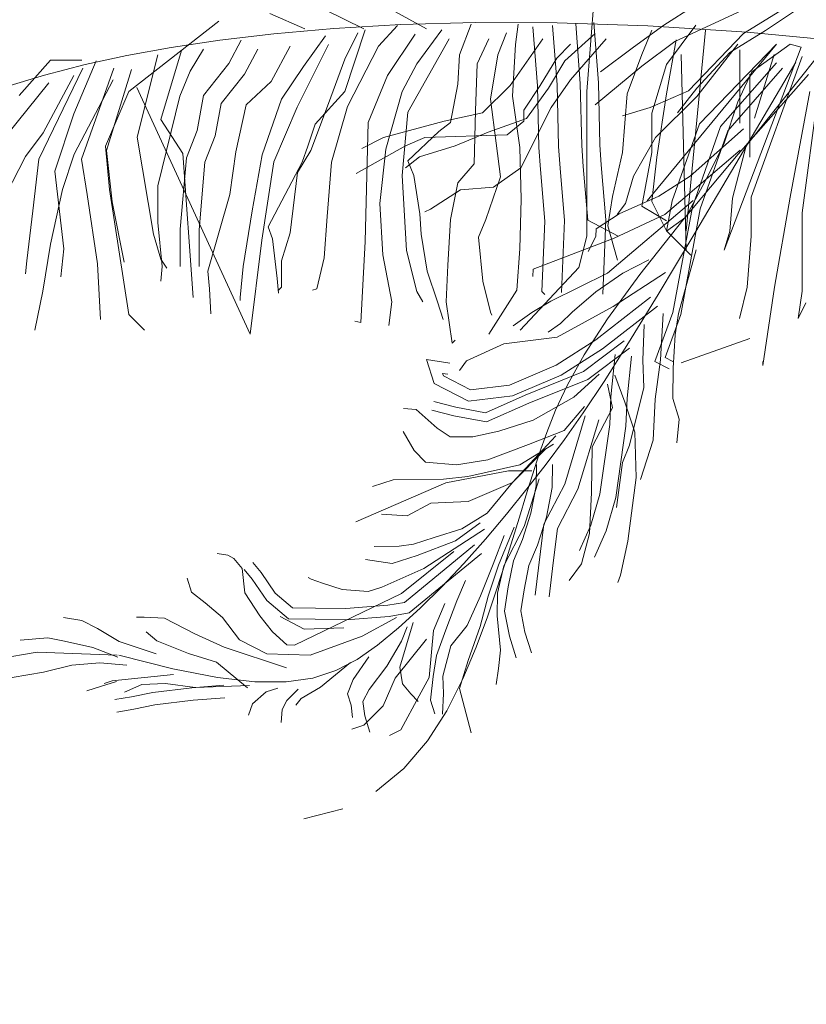
# Model space of a CAD drawing. Units: millimetres. Extents: x 595116 to 630915, y 909473 to 920225.
# Tile 34 of 134: x 629660.182 to 629667.505, y 919163.952 to 919173.119. Entities that reach past the tile are written whole.
import ezdxf

# ---------------------------------------------------------------- set-up
doc = ezdxf.new("R2010")
doc.units = ezdxf.units.MM
doc.layers.add('Dimension', color=3, linetype='Continuous', lineweight=18)
doc.layers.add('L-PLNT', color=85, linetype='Continuous', lineweight=13)
doc.styles.get("Standard").update_dxf_attribs({"font": 'arial.ttf'})
doc.dimstyles.new('ISO-25', dxfattribs={"dimtxt": 9, "dimasz": 6, "dimexe": 1.25, "dimexo": 0.625, "dimtad": 1, "dimlunit": 4, "dimtxsty": 'Standard', "dimcen": 2.5, "dimadec": 0, "dimazin": 0, "dimtfac": 1, "dimtmove": 0, "dimatfit": 3, "dimfxl": 1, "dimarcsym": 0})

# ---------------------------------------------------------------- blocks, each defined once
blk = doc.blocks.new('A$C4FB75ABC')
for p, q in [((2.1065, 2.3741), (2.087, 2.1315)), ((2.5983, 2.3508), (2.4757, 2.2759)), ((1.3881, 2.2867), (1.3008, 2.3255)), ((1.5337, 2.2867), (1.4367, 2.3352)), ((1.6891, 2.2867), (1.6017, 2.3352)), ((2.2781, 2.2963), (2.353, 2.344)), ((2.3054, 2.2555), (2.4825, 2.3372)), ((2.6119, 2.3372), (2.5302, 2.2827)), ((1.1746, 2.3061), (0.9513, 2.1315)), ((1.6258, 2.2976), (1.4598, 2.2878)), ((1.8099, 2.3026), (1.6258, 2.2976)), ((1.8004, 2.299), (1.7712, 2.2224)), ((2.0136, 2.3019), (1.8099, 2.3026)), ((1.9171, 2.299), (1.9098, 2.248)), ((2.2382, 2.2942), (2.0136, 2.3019)), ((2.0597, 2.2997), (2.0708, 2.1511)), ((2.1047, 2.3031), (2.1159, 2.1533)), ((2.2032, 2.2419), (2.2781, 2.2963)), ((2.3575, 2.296), (2.2846, 2.199)), ((1.3106, 2.2744), (1.1767, 2.2586)), ((1.4598, 2.2878), (1.3106, 2.2744)), ((1.5376, 2.2844), (1.4866, 2.1313)), ((1.5194, 2.2771), (1.4866, 2.2115)), ((1.6179, 2.2954), (1.5705, 2.2443)), ((1.6617, 2.2735), (1.5924, 2.1714)), ((1.7274, 2.2844), (1.6654, 2.2006)), ((1.8879, 2.2771), (1.8661, 2.2224)), ((1.9536, 2.2917), (1.9646, 2.1459)), ((2.0023, 2.2954), (2.0134, 2.1483)), ((2.1078, 2.2759), (2.0328, 2.2078)), ((2.2482, 2.2839), (2.2239, 2.2232)), ((2.4852, 2.2785), (2.2382, 2.2942)), ((2.3818, 2.2839), (2.3332, 1.7863)), ((2.4757, 2.2759), (2.3394, 2.1329)), ((2.5302, 2.2827), (2.4416, 2.2282)), ((2.7559, 2.2536), (2.4852, 2.2785)), ((1.1767, 2.2586), (1.0564, 2.241)), ((1.23, 2.2589), (1.1992, 2.2008)), ((1.4464, 2.2479), (1.3687, 2.0927)), ((1.4391, 2.2699), (1.3844, 2.1933)), ((1.7456, 2.2626), (1.6435, 2.0802)), ((1.8442, 2.2626), (1.815, 2.2006)), ((1.9783, 2.2623), (1.8966, 2.1465)), ((1.9098, 2.248), (1.9025, 2.1203)), ((2.0124, 2.2146), (2.0465, 2.2487)), ((2.135, 2.2623), (2.0465, 2.1602)), ((2.2236, 2.1942), (2.3054, 2.2555)), ((2.5574, 2.2487), (2.2372, 1.8605)), ((2.3089, 2.2596), (2.2846, 2.1261)), ((2.462, 2.2487), (2.3599, 2.1193)), ((2.3667, 2.0512), (2.5574, 2.2487)), ((2.6937, 2.2623), (2.4825, 1.9967)), ((2.5915, 2.2487), (2.4961, 2.1806)), ((2.6187, 2.2419), (2.5915, 2.2487)), ((1.0564, 2.241), (0.9464, 2.2213)), ((1.0231, 2.2224), (0.972, 2.0182)), ((1.0815, 2.2334), (1.0304, 2.062)), ((1.1363, 2.237), (1.1034, 2.1823)), ((1.2713, 2.237), (1.2384, 2.175)), ((1.3515, 2.2443), (1.3041, 2.1568)), ((1.5705, 2.2443), (1.4939, 2.0948)), ((1.7712, 2.2224), (1.7675, 2.1495)), ((1.8661, 2.2224), (1.8478, 2.113)), ((2.1214, 2.1806), (2.2032, 2.2419)), ((2.2239, 2.2232), (2.1875, 2.1261)), ((2.3211, 2.2232), (2.3332, 1.7378)), ((2.4416, 2.2282), (2.3599, 2.1397)), ((2.428, 1.738), (2.6187, 2.2419)), ((2.4668, 2.2354), (2.4668, 2.0533)), ((2.5518, 2.2232), (2.5032, 2.0655)), ((0.7572, 2.2091), (0.6795, 2.1218)), ((0.8429, 2.1986), (0.7422, 2.1723)), ((0.8348, 2.2091), (0.7572, 2.2091)), ((0.8699, 2.2079), (0.8151, 2.0766)), ((0.9464, 2.2213), (0.8429, 2.1986)), ((1.1992, 2.2008), (1.1362, 2.1221)), ((1.4866, 2.2115), (1.4464, 2.1021)), ((1.6654, 2.2006), (1.6289, 2.1313)), ((1.815, 2.2006), (1.8113, 2.0838)), ((1.9715, 2.1465), (2.0124, 2.2146)), ((2.0328, 2.2078), (1.992, 2.1397)), ((2.2846, 2.199), (2.2482, 2.0776)), ((2.5572, 2.203), (2.4187, 2.0449)), ((2.6056, 2.2048), (2.4676, 1.9701)), ((2.6209, 2.2188), (2.4948, 1.8695)), ((0.837, 2.1896), (0.7276, 1.9635)), ((0.9137, 2.1896), (0.8334, 1.9635)), ((0.9575, 2.186), (0.8954, 1.9854)), ((1.1034, 2.1823), (1.0779, 2.1203)), ((1.2384, 2.175), (1.18, 2.1021)), ((1.3844, 2.1933), (1.3297, 2.113)), ((2.1078, 2.0989), (2.2236, 2.1942)), ((2.5724, 2.1897), (2.4365, 2.0345)), ((2.4961, 2.1806), (2.462, 2.1057)), ((2.6368, 2.1742), (2.4628, 1.9766)), ((2.4911, 2.1747), (2.4911, 1.9684)), ((0.7422, 2.1723), (0.6405, 2.1416)), ((0.7531, 2.1531), (0.6473, 2.0218)), ((0.8151, 2.1714), (0.7385, 2.0291)), ((0.9125, 2.1606), (0.8154, 1.9763)), ((1.3041, 2.1568), (1.2421, 2.0984)), ((1.5924, 2.1714), (1.5449, 2.0547)), ((1.7675, 2.1495), (1.7493, 2.0547)), ((2.0465, 2.1602), (1.9988, 2.0921)), ((2.0708, 2.1511), (2.0745, 1.9975)), ((2.1159, 2.1533), (2.1196, 1.9995)), ((0.9513, 2.1315), (0.8931, 1.9957)), ((1.2522, 1.53), (0.9707, 2.1412)), ((1.4866, 2.1313), (1.4136, 2.051)), ((1.6289, 2.1313), (1.5887, 1.989)), ((1.8966, 2.1465), (1.8285, 2.0784)), ((1.9306, 2.0852), (1.9715, 2.1465)), ((1.992, 2.1397), (1.9375, 2.0648)), ((1.9646, 2.1459), (1.9682, 1.9927)), ((2.0134, 2.1483), (2.017, 1.9949)), ((2.087, 2.1315), (2.087, 1.7725)), ((2.1875, 2.1261), (2.1754, 1.9805)), ((2.3394, 2.1329), (2.244, 2.0921)), ((2.2846, 2.1261), (2.2604, 1.9684)), ((2.3599, 2.1397), (2.3122, 2.0784)), ((2.6404, 2.1315), (2.5918, 1.8695)), ((1.0779, 2.1203), (1.0231, 1.8978)), ((1.1362, 2.1221), (1.1203, 2.0346)), ((1.18, 2.1021), (1.1654, 2.0218)), ((1.3297, 2.113), (1.2822, 1.9744)), ((1.4464, 2.1021), (1.4026, 1.9854)), ((1.8478, 2.113), (1.8624, 2.0036)), ((1.9025, 2.1203), (1.9208, 1.9927)), ((2.3599, 2.1193), (2.2577, 2.0172)), ((2.462, 2.1057), (2.428, 2.0035)), ((2.6598, 2.1218), (2.6209, 1.8307)), ((0.8151, 2.0766), (0.7677, 1.9343)), ((1.2421, 2.0984), (1.2165, 1.9817)), ((1.3687, 2.0927), (1.3105, 1.9569)), ((1.4939, 2.0948), (1.4537, 1.9562)), ((1.6435, 2.0802), (1.6289, 1.9234)), ((1.8285, 2.0784), (1.7331, 2.058)), ((1.8113, 2.0838), (1.8077, 1.9526)), ((1.9988, 2.0921), (1.9238, 1.9422)), ((1.9306, 2.058), (1.9306, 2.0852)), ((2.244, 2.0921), (2.1759, 2.0716)), ((2.2482, 2.0776), (2.2482, 1.9805)), ((1.0304, 2.062), (1.0852, 1.9781)), ((1.5449, 2.0547), (1.5376, 1.7593)), ((1.7331, 2.058), (1.5832, 2.0172)), ((1.7493, 2.0547), (1.7201, 2.0328)), ((1.9375, 2.0648), (1.8421, 2.0308)), ((1.8898, 2.024), (1.9306, 2.058)), ((0.7385, 2.0291), (0.6947, 1.9708)), ((1.1203, 2.0346), (1.0939, 1.9669)), ((1.4136, 2.051), (1.3953, 1.9963)), ((1.7201, 2.0328), (1.6435, 1.9598)), ((1.8421, 2.0308), (1.7603, 1.9967)), ((2.2985, 1.8605), (2.3667, 2.0512)), ((2.4756, 2.0387), (2.3438, 1.9217)), ((2.4187, 2.0449), (2.3489, 1.8456)), ((2.4365, 2.0345), (2.3686, 1.8404)), ((0.972, 2.0182), (1.0122, 1.7775)), ((1.1654, 2.0218), (1.1399, 1.9562)), ((1.5832, 2.0172), (1.5287, 1.9899)), ((1.6377, 1.9967), (1.6854, 2.0172)), ((1.6854, 2.0172), (1.8898, 2.024)), ((1.8624, 2.0036), (1.8734, 1.9197)), ((2.2577, 2.0172), (2.2032, 1.9218)), ((2.428, 2.0035), (2.3871, 1.9218)), ((0.8931, 1.9957), (0.9028, 1.8889)), ((0.8954, 1.9854), (0.91, 1.8577)), ((1.2165, 1.9817), (1.2019, 1.876)), ((1.4026, 1.9854), (1.3698, 1.9307)), ((1.3953, 1.9963), (1.3807, 1.9562)), ((1.5151, 1.9286), (1.6377, 1.9967)), ((1.5887, 1.989), (1.5741, 1.8541)), ((1.7603, 1.9967), (1.6718, 1.9695)), ((1.9208, 1.9927), (1.9244, 1.865)), ((1.9682, 1.9927), (1.9719, 1.938)), ((2.017, 1.9949), (2.0206, 1.9417)), ((2.0745, 1.9975), (2.0779, 1.946)), ((2.1196, 1.9995), (2.1229, 1.9495)), ((2.1754, 1.9805), (2.1511, 1.8713)), ((2.2482, 1.9805), (2.2239, 1.847)), ((2.4673, 1.986), (2.2802, 1.8264)), ((2.4825, 1.9967), (2.4484, 1.8673)), ((0.6947, 1.9708), (0.629, 1.8431)), ((0.7276, 1.9635), (0.713, 1.8358)), ((0.8154, 1.9763), (0.7863, 1.8889)), ((0.8334, 1.9635), (0.848, 1.876)), ((1.0939, 1.9669), (1.0786, 1.7905)), ((1.0852, 1.9781), (1.1107, 1.6207)), ((1.1399, 1.9562), (1.1253, 1.7884)), ((1.2822, 1.9744), (1.2567, 1.8358)), ((1.3105, 1.9569), (1.2814, 1.7628)), ((1.3807, 1.9562), (1.2968, 1.7957)), ((1.4537, 1.9562), (1.4428, 1.8213)), ((1.6718, 1.9695), (1.6377, 1.9422)), ((1.6435, 1.9598), (1.6581, 1.9234)), ((2.2604, 1.9684), (2.2482, 1.8591)), ((2.4628, 1.9766), (2.3249, 1.8127)), ((2.4676, 1.9701), (2.3552, 1.7802)), ((0.7677, 1.9343), (0.7896, 1.741)), ((1.3698, 1.9307), (1.3515, 1.7811)), ((1.8077, 1.9526), (1.7675, 1.9051)), ((1.9238, 1.9422), (1.8557, 1.8946)), ((1.9719, 1.938), (1.9828, 1.8103)), ((2.0206, 1.9417), (2.0317, 1.8114)), ((2.0779, 1.946), (2.0893, 1.8127)), ((2.1229, 1.9495), (2.1345, 1.8136)), ((1.6289, 1.9234), (1.6398, 1.7374)), ((1.6581, 1.9234), (1.6727, 1.8285)), ((1.7675, 1.9051), (1.7493, 1.814)), ((1.8734, 1.9197), (1.8369, 1.814)), ((2.2032, 1.9218), (2.1827, 1.8537)), ((2.3438, 1.9217), (2.2657, 1.8718)), ((2.3871, 1.9218), (2.3326, 1.8197)), ((0.7863, 1.8889), (0.7572, 1.7531)), ((0.9028, 1.8889), (0.9513, 1.5785)), ((1.0231, 1.8978), (1.0231, 1.8067)), ((1.7739, 1.8878), (1.699, 1.8401)), ((1.8557, 1.8946), (1.7739, 1.8878)), ((0.848, 1.876), (0.8735, 1.7045)), ((0.91, 1.8577), (0.9392, 1.7082)), ((1.2019, 1.876), (1.1472, 1.6863)), ((1.9244, 1.865), (1.9208, 1.741)), ((2.3505, 1.8613), (2.1386, 1.6813)), ((2.1511, 1.8713), (2.1389, 1.7985)), ((2.2657, 1.8718), (2.167, 1.8279)), ((2.2482, 1.8591), (2.2846, 1.7863)), ((2.2849, 1.7856), (2.2985, 1.8605)), ((2.4484, 1.8673), (2.4416, 1.7856)), ((2.4948, 1.8695), (2.4948, 1.7725)), ((2.5918, 1.8695), (2.553, 1.6464)), ((0.713, 1.8358), (0.6984, 1.7118)), ((1.2567, 1.8358), (1.2348, 1.6973)), ((1.5741, 1.8541), (1.5814, 1.7264)), ((1.699, 1.8401), (1.6854, 1.8333)), ((2.1827, 1.8537), (2.1623, 1.8265)), ((2.2239, 1.847), (2.2846, 1.8106)), ((2.3489, 1.8456), (2.3004, 1.5838)), ((2.3686, 1.8404), (2.32, 1.5785)), ((1.4428, 1.8213), (1.4355, 1.7191)), ((1.6727, 1.8285), (1.6763, 1.7775)), ((1.7493, 1.814), (1.742, 1.7009)), ((1.8369, 1.814), (1.8186, 1.7702)), ((1.9828, 1.8103), (1.9755, 1.6352)), ((2.0317, 1.8114), (2.0243, 1.6332)), ((2.0893, 1.8127), (2.1647, 1.7725)), ((2.167, 1.8279), (2.1099, 1.791)), ((2.1345, 1.8136), (2.1268, 1.6289)), ((2.2802, 1.8264), (2.1549, 1.7678)), ((2.3249, 1.8127), (2.2184, 1.678)), ((2.3326, 1.8197), (2.2849, 1.7856)), ((2.6209, 1.8307), (2.6209, 1.6367)), ((1.0231, 1.8067), (1.0341, 1.6973)), ((1.0786, 1.7905), (1.0786, 1.6973)), ((1.1253, 1.7884), (1.1253, 1.7665)), ((1.2968, 1.7957), (1.3078, 1.7665)), ((2.1099, 1.791), (2.1096, 1.7722)), ((2.1389, 1.7985), (2.1632, 1.7135)), ((2.2846, 1.7863), (2.3453, 1.7256)), ((2.4416, 1.7856), (2.428, 1.738)), ((1.0122, 1.7775), (1.0304, 1.7155)), ((1.1253, 1.7665), (1.1253, 1.7301)), ((1.2814, 1.7628), (1.2522, 1.53)), ((1.3078, 1.7665), (1.3187, 1.6681)), ((1.3515, 1.7811), (1.3297, 1.7118)), ((1.5376, 1.7593), (1.5267, 1.5587)), ((1.6763, 1.7775), (1.6909, 1.6863)), ((1.8186, 1.7702), (1.8296, 1.6608)), ((2.1549, 1.7678), (1.9538, 1.6913)), ((2.087, 1.7725), (2.0676, 1.6949)), ((2.1096, 1.7722), (2.0903, 1.7347)), ((2.3552, 1.7802), (2.2641, 1.6283)), ((2.4948, 1.7725), (2.485, 1.6464)), ((0.7572, 1.7531), (0.7377, 1.6367)), ((0.7896, 1.741), (0.7823, 1.6717)), ((1.6398, 1.7374), (1.6654, 1.6352)), ((1.9208, 1.741), (1.9135, 1.6389)), ((2.3582, 1.7386), (2.3145, 1.5808)), ((0.6984, 1.7118), (0.6947, 1.679)), ((1.0304, 1.7155), (1.045, 1.6936)), ((1.1253, 1.7301), (1.1253, 1.6973)), ((1.3297, 1.7118), (1.3297, 1.6462)), ((1.4355, 1.7191), (1.4172, 1.6425)), ((1.5814, 1.7264), (1.6033, 1.6097)), ((2.2409, 1.7138), (2.1763, 1.6807)), ((0.8735, 1.7045), (0.8808, 1.566)), ((1.0341, 1.6973), (1.0304, 1.6608)), ((1.1472, 1.6863), (1.1509, 1.6425)), ((1.2348, 1.6973), (1.2275, 1.6207)), ((1.6909, 1.6863), (1.7164, 1.6097)), ((1.742, 1.7009), (1.7383, 1.6097)), ((2.0676, 1.6949), (1.922, 1.5397)), ((1.9538, 1.6913), (1.9536, 1.6725)), ((1.3187, 1.6681), (1.3224, 1.6316)), ((1.8296, 1.6608), (1.8478, 1.5842)), ((2.1386, 1.6813), (1.998, 1.6115)), ((2.1763, 1.6807), (2.1096, 1.6345)), ((2.2184, 1.678), (2.1385, 1.568)), ((2.2819, 1.6831), (2.1525, 1.5981)), ((0.7377, 1.6367), (0.7183, 1.5397)), ((1.1509, 1.6425), (1.1545, 1.5805)), ((1.3297, 1.6462), (1.3224, 1.6389)), ((1.4172, 1.6425), (1.4063, 1.6389)), ((1.9135, 1.6389), (1.8444, 1.53)), ((2.485, 1.6464), (2.4656, 1.5688)), ((2.553, 1.6464), (2.5239, 1.4523)), ((2.6209, 1.6367), (2.6112, 1.5688)), ((1.2275, 1.6207), (1.2275, 1.6134)), ((1.6654, 1.6352), (1.68, 1.6097)), ((1.9755, 1.6352), (1.9828, 1.628)), ((2.1096, 1.6345), (2.0504, 1.5844)), ((2.2452, 1.6213), (2.1098, 1.5157)), ((2.2641, 1.6283), (2.1904, 1.5079)), ((1.6033, 1.6097), (1.596, 1.5514)), ((1.7164, 1.6097), (1.731, 1.566)), ((1.7383, 1.6097), (1.7529, 1.5076)), ((1.998, 1.6115), (1.9504, 1.5839)), ((2.1525, 1.5981), (2.0137, 1.5227)), ((2.2623, 1.5995), (2.1258, 1.493)), ((2.6112, 1.5688), (2.6307, 1.6076)), ((0.9513, 1.5785), (0.9901, 1.5397)), ((1.8478, 1.5842), (1.8515, 1.5769)), ((1.9504, 1.5839), (1.9047, 1.5506)), ((2.0504, 1.5844), (2.0217, 1.5565)), ((2.1385, 1.568), (2.0803, 1.4783)), ((2.3004, 1.5838), (2.256, 1.4617)), ((2.2767, 1.5813), (2.2695, 1.4664)), ((2.32, 1.5785), (2.2812, 1.4717)), ((2.3145, 1.5808), (2.3062, 1.5281)), ((1.5267, 1.5587), (1.5121, 1.5623)), ((2.0217, 1.5565), (1.9912, 1.5343)), ((2.2292, 1.5537), (2.2261, 1.4651)), ((1.7529, 1.5076), (1.7602, 1.5149)), ((2.0137, 1.5227), (1.8814, 1.5056)), ((2.1098, 1.5157), (2.0109, 1.453)), ((2.3062, 1.5281), (2.3013, 1.4452)), ((2.4911, 1.5193), (2.3211, 1.4586)), ((1.8814, 1.5056), (1.7884, 1.4636)), ((2.1258, 1.493), (2.0238, 1.4284)), ((2.1796, 1.5129), (2.0785, 1.437)), ((2.1927, 1.4954), (2.0894, 1.4177)), ((2.1904, 1.5079), (2.1298, 1.4122)), ((1.7084, 1.4073), (1.6895, 1.4666)), ((1.6895, 1.4666), (1.747, 1.4576)), ((2.0803, 1.4783), (2.039, 1.4043)), ((2.1578, 1.4791), (2.1468, 1.3743)), ((2.1979, 1.4749), (2.187, 1.3714)), ((2.2695, 1.4664), (2.2568, 1.3685)), ((2.2812, 1.4717), (2.3006, 1.462)), ((1.7884, 1.4636), (1.7711, 1.4393)), ((2.0109, 1.453), (1.8951, 1.4036)), ((2.2261, 1.4651), (2.2289, 1.3972)), ((2.256, 1.4617), (2.2916, 1.4439)), ((2.3013, 1.4452), (2.3002, 1.3698)), ((2.5239, 1.4523), (2.5239, 1.462)), ((1.7313, 1.4266), (1.7295, 1.4323)), ((1.7295, 1.4323), (1.7427, 1.4302)), ((1.7987, 1.3918), (1.7313, 1.4266)), ((2.0238, 1.4284), (1.9024, 1.3766)), ((2.0785, 1.437), (1.9344, 1.3786)), ((2.0894, 1.4177), (1.9429, 1.3584)), ((2.1181, 1.4308), (2.055, 1.3732)), ((2.1569, 1.4277), (2.1816, 1.3609)), ((1.7936, 1.3632), (1.7084, 1.4073)), ((1.8951, 1.4036), (1.7987, 1.3918)), ((2.039, 1.4043), (2.0098, 1.3416)), ((2.1298, 1.4122), (2.0784, 1.3347)), ((2.1385, 1.406), (2.1509, 1.3473)), ((2.2289, 1.3972), (2.1929, 1.2544)), ((1.9024, 1.3766), (1.7936, 1.3632)), ((1.9344, 1.3786), (1.8357, 1.3347)), ((2.055, 1.3732), (1.9542, 1.3161)), ((2.1468, 1.3743), (2.1439, 1.3053)), ((2.187, 1.3714), (2.1842, 1.3016)), ((2.2568, 1.3685), (2.2516, 1.2668)), ((2.3002, 1.3698), (2.3165, 1.3187)), ((1.6641, 1.3427), (1.6321, 1.345)), ((1.7623, 1.3489), (1.7078, 1.3628)), ((1.8357, 1.3347), (1.7623, 1.3489)), ((1.9429, 1.3584), (1.8383, 1.3119)), ((2.0811, 1.3502), (2.0312, 1.2905)), ((2.1509, 1.3473), (2.1005, 1.25)), ((2.1816, 1.3609), (2.2062, 1.287)), ((1.7163, 1.2967), (1.6641, 1.3427)), ((1.7575, 1.3275), (1.7024, 1.3416)), ((1.8383, 1.3119), (1.7575, 1.3275)), ((2.0098, 1.3416), (1.9878, 1.2857)), ((2.0784, 1.3347), (2.0319, 1.2687)), ((2.0829, 1.3276), (2.0324, 1.158)), ((1.7481, 1.2755), (1.7163, 1.2967)), ((1.9542, 1.3161), (1.869, 1.289)), ((2.1165, 1.3176), (2.065, 1.1449)), ((2.1439, 1.3053), (2.1195, 1.1332)), ((2.1842, 1.3016), (2.1591, 1.1247)), ((2.3165, 1.3187), (2.31, 1.2603)), ((1.6589, 1.2409), (1.6313, 1.2885)), ((1.8046, 1.2748), (1.7481, 1.2755)), ((1.869, 1.289), (1.8046, 1.2748)), ((2.0103, 1.2776), (1.903, 1.1622)), ((2.0312, 1.2905), (1.9421, 1.2559)), ((1.9878, 1.2857), (1.9691, 1.2327)), ((2.2062, 1.287), (2.2097, 1.1745)), ((1.9421, 1.2559), (1.8416, 1.2177)), ((2.0043, 1.257), (1.9206, 1.2053)), ((2.0319, 1.2687), (1.9864, 1.2075)), ((2.1005, 1.25), (2.0989, 1.1369)), ((2.1929, 1.2544), (2.1754, 1.2112)), ((2.2516, 1.2668), (2.22, 1.1691)), ((1.6868, 1.2123), (1.6589, 1.2409)), ((1.9834, 1.244), (1.903, 1.1622)), ((1.9691, 1.2327), (1.952, 1.1808)), ((1.7641, 1.2056), (1.6868, 1.2123)), ((1.8416, 1.2177), (1.7641, 1.2056)), ((1.9206, 1.2053), (1.792, 1.1769)), ((1.9864, 1.2075), (1.9386, 1.1458)), ((1.9621, 1.2066), (1.9614, 1.1536)), ((2.0017, 1.2061), (2.001, 1.1495)), ((2.1754, 1.2112), (2.1606, 1.1002)), ((1.792, 1.1769), (1.7315, 1.1702)), ((1.7376, 1.1613), (1.8929, 1.1904)), ((1.8929, 1.1904), (1.9511, 1.1904)), ((1.952, 1.1808), (1.9358, 1.129)), ((2.2097, 1.1745), (2.1886, 1.0162)), ((1.5143, 1.0642), (1.7376, 1.1613)), ((1.607, 1.1681), (1.5558, 1.1518)), ((1.7315, 1.1702), (1.607, 1.1681)), ((1.903, 1.1622), (1.793, 1.1147)), ((1.903, 1.1622), (1.8397, 1.0857)), ((1.9692, 1.1707), (1.9317, 1.0524)), ((1.9614, 1.1536), (1.9482, 1.0859)), ((2.0324, 1.158), (1.9806, 1.0581)), ((2.001, 1.1495), (1.9867, 1.0762)), ((1.9386, 1.1458), (1.8882, 1.0835)), ((1.9358, 1.129), (1.9198, 1.076)), ((2.065, 1.1449), (2.0146, 1.0475)), ((2.0989, 1.1369), (2.0937, 1.0351)), ((2.1195, 1.1332), (2.0972, 1.056)), ((2.1591, 1.1247), (2.1353, 1.0421)), ((1.7005, 1.1103), (1.6416, 1.079)), ((1.793, 1.1147), (1.7005, 1.1103)), ((1.6416, 1.079), (1.5775, 1.0837)), ((1.8397, 1.0857), (1.7769, 1.047)), ((1.8882, 1.0835), (1.8359, 1.0215)), ((1.9198, 1.076), (1.903, 1.0206)), ((1.9482, 1.0859), (1.9278, 1.0204)), ((1.9867, 1.0762), (1.965, 1.0067)), ((1.8224, 1.0615), (1.7614, 1.017)), ((1.9071, 1.0509), (1.8681, 0.9571)), ((1.9317, 1.0524), (1.8813, 0.9551)), ((1.9806, 1.0581), (1.9586, 0.8825)), ((2.0972, 1.056), (2.0692, 0.9929)), ((1.8335, 1.0462), (1.6831, 0.9483)), ((1.7769, 1.047), (1.7087, 1.0253)), ((1.8823, 1.0305), (1.8549, 0.9592)), ((2.0146, 1.0475), (2.004, 0.9628)), ((2.0937, 1.0351), (2.0738, 0.96)), ((2.1353, 1.0421), (2.1061, 0.9765)), ((1.6216, 1.0039), (1.5594, 1.0028)), ((1.6576, 1.009), (1.6216, 1.0039)), ((1.8084, 1.007), (1.6348, 0.8642)), ((1.7087, 1.0253), (1.6576, 1.009)), ((1.7614, 1.017), (1.6666, 0.9806)), ((1.8359, 1.0215), (1.7823, 0.9612)), ((1.903, 1.0206), (1.8847, 0.9618)), ((1.9278, 1.0204), (1.9055, 0.9679)), ((1.965, 1.0067), (1.9435, 0.9561)), ((2.1886, 1.0162), (2.171, 0.9318)), ((1.1969, 0.9814), (1.1705, 0.9855)), ((1.2119, 0.9737), (1.1969, 0.9814)), ((1.6666, 0.9806), (1.6041, 0.9607)), ((1.7573, 0.9907), (1.6276, 0.8869)), ((1.8259, 0.9857), (1.6466, 0.8382)), ((1.2323, 0.9489), (1.2119, 0.9737)), ((1.2793, 0.9388), (1.2589, 0.9636)), ((1.6041, 0.9607), (1.5382, 0.9711)), ((1.7823, 0.9612), (1.7281, 0.9036)), ((1.8549, 0.9592), (1.8236, 0.8804)), ((1.8681, 0.9571), (1.8425, 0.8802)), ((1.8847, 0.9618), (1.8642, 0.8983)), ((1.8813, 0.9551), (1.8652, 0.8874)), ((1.9055, 0.9679), (1.8924, 0.9029)), ((1.9435, 0.9561), (1.9314, 0.8959)), ((2.004, 0.9628), (1.9934, 0.8781)), ((2.0738, 0.96), (2.043, 0.9189)), ((1.239, 0.8884), (1.2323, 0.9489)), ((1.2572, 0.9222), (1.2376, 0.9461)), ((1.3144, 0.8874), (1.2793, 0.9388)), ((1.6831, 0.9483), (1.5787, 0.9026)), ((2.171, 0.9318), (2.164, 0.9142)), ((1.107, 0.8902), (1.0961, 0.9243)), ((1.2938, 0.8688), (1.2572, 0.9222)), ((1.4036, 0.922), (1.3961, 0.9259)), ((1.4317, 0.9122), (1.4036, 0.922)), ((1.4805, 0.8964), (1.4317, 0.9122)), ((1.7864, 0.9186), (1.765, 0.868)), ((1.1405, 0.8634), (1.107, 0.8902)), ((1.2759, 0.8314), (1.239, 0.8884)), ((1.3573, 0.851), (1.3144, 0.8874)), ((1.6276, 0.8869), (1.3617, 0.7585)), ((1.5446, 0.8918), (1.4805, 0.8964)), ((1.5787, 0.9026), (1.5446, 0.8918)), ((1.7281, 0.9036), (1.6739, 0.8498)), ((1.8236, 0.8804), (1.7906, 0.8073)), ((1.8425, 0.8802), (1.8226, 0.805)), ((1.8642, 0.8983), (1.8405, 0.829)), ((1.8652, 0.8874), (1.8644, 0.8308)), ((1.8924, 0.9029), (1.8829, 0.8424)), ((1.9314, 0.8959), (1.9231, 0.8432)), ((1.1834, 0.827), (1.1405, 0.8634)), ((1.347, 0.8236), (1.2938, 0.8688)), ((1.5932, 0.8572), (1.4893, 0.8492)), ((1.6348, 0.8642), (1.5932, 0.8572)), ((1.7347, 0.8614), (1.7065, 0.7946)), ((1.765, 0.868), (1.7376, 0.7967)), ((1.3074, 0.7913), (1.2759, 0.8314)), ((1.4139, 0.8502), (1.3573, 0.851)), ((1.4893, 0.8492), (1.4139, 0.8502)), ((1.6466, 0.8382), (1.5965, 0.8298)), ((1.6739, 0.8498), (1.6204, 0.8011)), ((1.8644, 0.8308), (1.8727, 0.7459)), ((1.8829, 0.8424), (1.8952, 0.7804)), ((1.9231, 0.8432), (1.9337, 0.7903)), ((0.8346, 0.8198), (0.7888, 0.827)), ((0.8736, 0.7996), (0.8346, 0.8198)), ((0.9891, 0.8277), (0.9703, 0.828)), ((1.04, 0.8252), (0.9891, 0.8277)), ((1.1149, 0.7864), (1.04, 0.8252)), ((1.226, 0.7717), (1.1834, 0.827)), ((1.3863, 0.7981), (1.3265, 0.8298)), ((1.4135, 0.8227), (1.347, 0.8236)), ((1.4902, 0.8216), (1.4135, 0.8227)), ((1.5965, 0.8298), (1.4902, 0.8216)), ((1.6154, 0.8267), (1.5299, 0.7807)), ((1.6567, 0.8148), (1.6231, 0.704)), ((1.7906, 0.8073), (1.7502, 0.757)), ((1.8405, 0.829), (1.8129, 0.7535)), ((0.9273, 0.7678), (0.8736, 0.7996)), ((1.0204, 0.7689), (0.9943, 0.7918)), ((1.188, 0.7534), (1.1149, 0.7864)), ((1.3428, 0.7588), (1.3074, 0.7913)), ((1.4848, 0.8016), (1.3863, 0.7981)), ((1.6204, 0.8011), (1.5682, 0.7585)), ((1.6415, 0.8037), (1.6278, 0.7681)), ((1.7065, 0.7946), (1.696, 0.6785)), ((1.7376, 0.7967), (1.7141, 0.733)), ((1.8226, 0.805), (1.7931, 0.7206)), ((1.9337, 0.7903), (1.9499, 0.7392)), ((0.7503, 0.7767), (0.6814, 0.7711)), ((0.7912, 0.768), (0.7503, 0.7767)), ((0.8615, 0.7523), (0.7912, 0.768)), ((1.0187, 0.737), (0.9273, 0.7678)), ((1.0992, 0.7376), (1.0204, 0.7689)), ((1.2935, 0.7368), (1.226, 0.7717)), ((1.3617, 0.7585), (1.3428, 0.7588)), ((1.5299, 0.7807), (1.4009, 0.7335)), ((1.5682, 0.7585), (1.5172, 0.7231)), ((1.6278, 0.7681), (1.5911, 0.7064)), ((1.6891, 0.7732), (1.6114, 0.6762)), ((1.8952, 0.7804), (1.9122, 0.7271)), ((0.7236, 0.7411), (0.5379, 0.7092)), ((0.9219, 0.7334), (0.7236, 0.7411)), ((0.9235, 0.7285), (0.8615, 0.7523)), ((1.0599, 0.6997), (0.9265, 0.7333)), ((1.1687, 0.7159), (1.0992, 0.7376)), ((1.342, 0.7022), (1.188, 0.7534)), ((1.4009, 0.7335), (1.2935, 0.7368)), ((1.7141, 0.733), (1.7058, 0.6803)), ((1.7502, 0.757), (1.7303, 0.6818)), ((1.8129, 0.7535), (1.7799, 0.6746)), ((1.8727, 0.7459), (1.8683, 0.7007)), ((0.8101, 0.7087), (0.7393, 0.6917)), ((0.879, 0.7143), (0.8101, 0.7087)), ((0.9462, 0.7085), (0.879, 0.7143)), ((1.2451, 0.6526), (1.1687, 0.7159)), ((1.5006, 0.7151), (1.4262, 0.6539)), ((1.5172, 0.7231), (1.4647, 0.6957)), ((1.5461, 0.7296), (1.5076, 0.6736)), ((1.7931, 0.7206), (1.7714, 0.6511)), ((0.7393, 0.6917), (0.6621, 0.678)), ((1.0623, 0.6856), (0.9095, 0.6697)), ((1.1712, 0.6779), (1.0599, 0.6997)), ((1.4647, 0.6957), (1.4072, 0.6768)), ((1.5911, 0.7064), (1.5469, 0.6485)), ((1.6231, 0.704), (1.6301, 0.6625)), ((1.8683, 0.7007), (1.8621, 0.6612)), ((0.9209, 0.6684), (0.8811, 0.6557)), ((0.9095, 0.6697), (0.8898, 0.6634)), ((0.9832, 0.6605), (0.9403, 0.6414)), ((1.0423, 0.6629), (0.9832, 0.6605)), ((1.1159, 0.6537), (1.0423, 0.6629)), ((1.2639, 0.6673), (1.1712, 0.6779)), ((1.3414, 0.6671), (1.2639, 0.6673)), ((1.4072, 0.6768), (1.3414, 0.6671)), ((1.5076, 0.6736), (1.4939, 0.6379)), ((1.6114, 0.6762), (1.5823, 0.6082)), ((1.6301, 0.6625), (1.6505, 0.6377)), ((1.696, 0.6785), (1.6713, 0.6328)), ((1.7058, 0.6803), (1.6993, 0.6219)), ((1.7303, 0.6818), (1.7316, 0.6384)), ((1.7799, 0.6746), (1.74, 0.5958)), ((0.8811, 0.6557), (0.847, 0.6449)), ((1.011, 0.6408), (0.9581, 0.6302)), ((1.1074, 0.6526), (1.011, 0.6408)), ((1.1867, 0.6591), (1.1074, 0.6526)), ((1.2504, 0.6584), (1.1159, 0.6537)), ((1.2921, 0.6426), (1.2578, 0.6129)), ((1.3206, 0.6516), (1.2921, 0.6426)), ((1.3714, 0.649), (1.3428, 0.6211)), ((1.4262, 0.6539), (1.3787, 0.6263)), ((1.4939, 0.6379), (1.5029, 0.6095)), ((1.5469, 0.6485), (1.5314, 0.6186)), ((1.6505, 0.6377), (1.6691, 0.6186)), ((1.7316, 0.6384), (1.729, 0.5876)), ((1.7714, 0.6511), (1.8, 0.5413)), ((0.9581, 0.6302), (0.9165, 0.6232)), ((1.1106, 0.6216), (1.016, 0.61)), ((1.1893, 0.628), (1.1106, 0.6216)), ((1.2578, 0.6129), (1.2479, 0.5847)), ((1.3428, 0.6211), (1.3311, 0.5987)), ((1.3787, 0.6263), (1.3652, 0.6095)), ((1.5314, 0.6186), (1.5365, 0.5827)), ((1.6713, 0.6328), (1.6256, 0.5484)), ((1.6993, 0.6219), (1.7101, 0.5878)), ((0.9632, 0.5994), (0.9216, 0.5925)), ((1.016, 0.61), (0.9632, 0.5994)), ((1.3311, 0.5987), (1.3288, 0.5666)), ((1.5029, 0.6095), (1.5063, 0.5793)), ((1.5823, 0.6082), (1.5337, 0.5597)), ((1.74, 0.5958), (1.6917, 0.5207)), ((1.5365, 0.5827), (1.5492, 0.5429)), ((1.5337, 0.5597), (1.5046, 0.55)), ((1.6256, 0.5484), (1.5974, 0.5343)), ((1.6917, 0.5207), (1.6336, 0.4527)), ((1.6336, 0.4527), (1.5642, 0.3956)), ((1.4819, 0.3527), (1.3853, 0.3277))]:
    blk.add_line(p, q)
blk = doc.blocks.new('*D216')
at = {"layer": 'Defpoints', "color": 0, "transparency": 16777216}
for p in [(629743.5408, 919411.9276), (629505.0408, 919411.8279), (629743.5408, 918832.3776)]:
    blk.add_point(p, dxfattribs=at)
at = {"layer": 'Dimension', "color": 0, "lineweight": -2, "transparency": 16777216}
for p, q in [((629743.5408, 919411.3026), (629743.5408, 918831.1276)), ((629505.0408, 919411.2029), (629505.0408, 918831.1276)), ((629511.0408, 918832.3776), (629737.5408, 918832.3776))]:
    blk.add_line(p, q, dxfattribs=at)
at = {"layer": 'Dimension', "color": 0, "transparency": 16777216}
for points in [[(629511.0408, 918833.3776), (629511.0408, 918831.3776), (629505.0408, 918832.3776)], [(629737.5408, 918833.3776), (629737.5408, 918831.3776), (629743.5408, 918832.3776)]]:
    blk.add_solid(points, dxfattribs=at)
at = {"layer": 'Dimension', "color": 0, "transparency": 16777216, "insert": (629624.2908, 918837.656), "char_height": 9, "attachment_point": 5}
blk.add_mtext('19\'-10 1/2"', dxfattribs=at)

msp = doc.modelspace()

# ---------------------------------------------------------------- block references
at = {"layer": 'L-PLNT', "xscale": 3.753413438031968, "yscale": 3.753413438031968, "zscale": 3.753413438031968}
msp.add_blockref('A$C4FB75ABC', (629657.6275, 919164.4492), dxfattribs=at)

# ---------------------------------------------------------------- dimensions: what is measured, and where the dimension line sits
at = {"layer": 'Dimension'}
dim = msp.add_linear_dim(base=(629743.5408, 918832.3776), p1=(629505.0408, 919411.8279), p2=(629743.5408, 919411.9276), dimstyle='ISO-25', override={"dimdec": 1, "dimlfac": 1, "dimrnd": 0, "dimzin": 1, "dimdsep": 46, "dimlunit": 4, "dimfrac": 2}, dxfattribs=at)
dim.commit()
dim.dimension.update_dxf_attribs({"geometry": '*D216', "text_midpoint": (629624.2908, 918837.656)})

doc.saveas('drawing.dxf')
